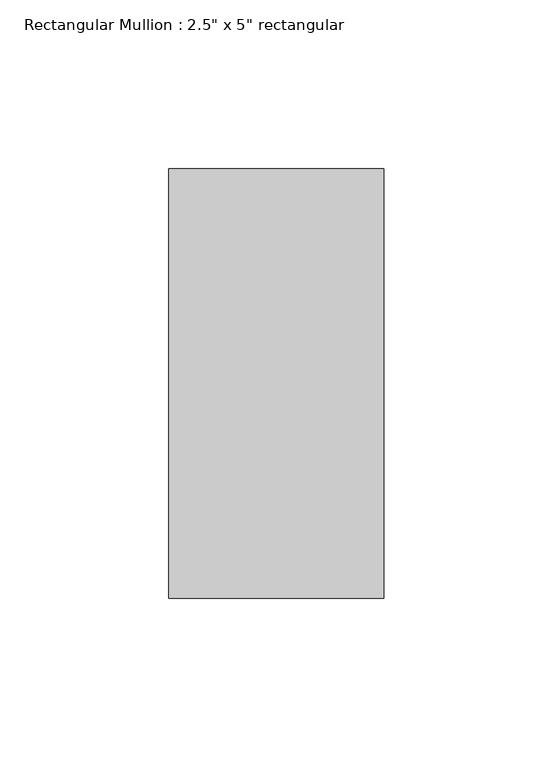
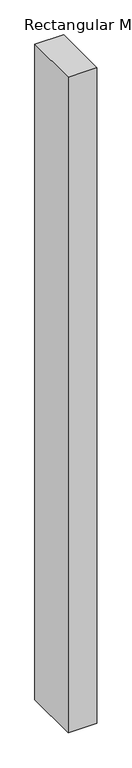
"""IFC4 building model written with IfcOpenShell, lengths in millimetres: member geometry."""

from ifc_helpers import new_model, si_unit, frame, origin, place, context, project, spatial, polyline, outline, extrude, source, transform, mapped, element, save


def member_b984fe7d(model_context):
    return source(origin(), model_context, "Body", "SweptSolid", [
        extrude(outline(polyline([(31.75, 63.5), (31.75, -63.5), (-31.75, -63.5), (-31.75, 63.5), (31.75, 63.5)])), frame((0.0, 0.0, -1531.3368617), z_axis=(0.0, 0.0, 1.0), x_axis=(1.0, 0.0, 0.0)), (0.0, 0.0, 1.0), 1531.3368617),
    ])


if __name__ == "__main__":
    model = new_model("IFC4")
    model_context = context("Model", 3, world=origin())
    ifc_project = project(units=[si_unit("LENGTHUNIT", "METRE", prefix="MILLI")], contexts=[model_context])
    site = spatial("IfcSite", under=ifc_project)
    building = spatial("IfcBuilding", under=site)
    placement = place(None, origin())
    member_shape = member_b984fe7d(model_context)
    element("IfcMember", 1, ObjectType="Rectangular Mullion : 2.5\" x 5\" rectangular", at=placement, inside=building, context=model_context, shape_type="MappedRepresentation", body=[
        mapped(member_shape, transform((0.0, 0.0, 0.0), x_axis=(1.0, 0.0, 0.0), y_axis=(0.0, 1.0, 0.0), z_axis=(0.0, 0.0, 1.0))),
    ])
    save(model, "model.ifc")

# Revit data of these elements
# Type "Rectangular Mullion : 2.5\" x 5\" rectangular"
#   built-in parameter 1007304 = 0.416667 (stored number, unit not read)
#   built-in parameter 1007301 = 0.104167 (stored number, unit not read)
#   built-in parameter 1007300 = 0.104167 (stored number, unit not read)
# Element 1 (IfcMember, "Rectangular Mullion : 2.5\" x 5\" rectangular")
#   Materials on its faces: "Aluminum"
# Materials
#   "Aluminum": class "Metal", colour RGB 247 247 247, transparency 0, Description = "Aluminum 6061", Cost = 0
